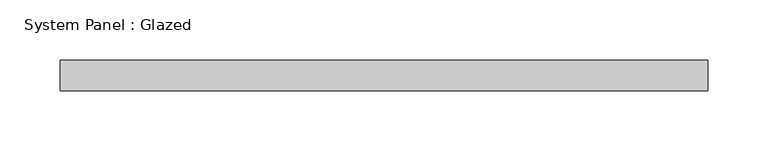
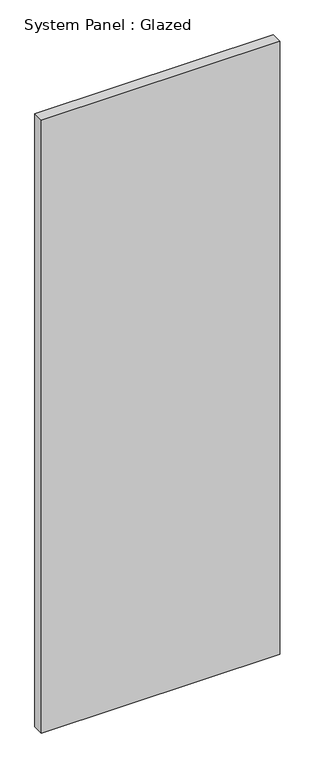
"""IFC4 building model written with IfcOpenShell, lengths in millimetres: plate geometry, System Panel : Glazed."""

from ifc_helpers import new_model, si_unit, origin, origin_with_axes, place, context, project, spatial, polyline, outline, extrude, source, transform, mapped, element, save


def system_panel_glazed_cb6b9410(model_context):
    return source(origin(), model_context, "Body", "SweptSolid", [
        extrude(outline(polyline([(269.875, 19.05), (-269.875, 19.05), (-269.875, 44.45), (269.875, 44.45), (269.875, 19.05)])), origin_with_axes(), (0.0, 0.0, 1.0), 1467.6445261),
    ])


if __name__ == "__main__":
    model = new_model("IFC4")
    model_context = context("Model", 3, world=origin())
    ifc_project = project(units=[si_unit("LENGTHUNIT", "METRE", prefix="MILLI")], contexts=[model_context])
    site = spatial("IfcSite", under=ifc_project)
    building = spatial("IfcBuilding", under=site)
    placement = place(None, origin())
    system_panel_glazed_shape = system_panel_glazed_cb6b9410(model_context)
    element("IfcPlate", 1, ObjectType="System Panel : Glazed", at=placement, inside=building, context=model_context, shape_type="MappedRepresentation", body=[
        mapped(system_panel_glazed_shape, transform((0.0, 0.0, 0.0), x_axis=(1.0, 0.0, 0.0), y_axis=(0.0, 1.0, 0.0), z_axis=(0.0, 0.0, 1.0))),
    ])
    save(model, "model.ifc")

# Revit data of these elements
# Type "System Panel : Glazed"
#   Construction Type Id = "GSP4R"
#   Analytic Construction = "1/8 in Pilkington single glazing"
#   Visual Light Transmittance = 0.9
#   Solar Heat Gain Coefficient = 0.86
#   Heat Transfer Coefficient (U) = 1.18115 BTU/(h·ft²·°F)
#   Define Thermal Properties by = 1
# Element 1 (IfcPlate, "System Panel : Glazed")
#   Materials on its faces: "Glass"
# Materials
#   "Glass": class "Glass", colour RGB 0 128 192, transparency 0.75, Description = "Soda Lime Glass", Cost = 0
